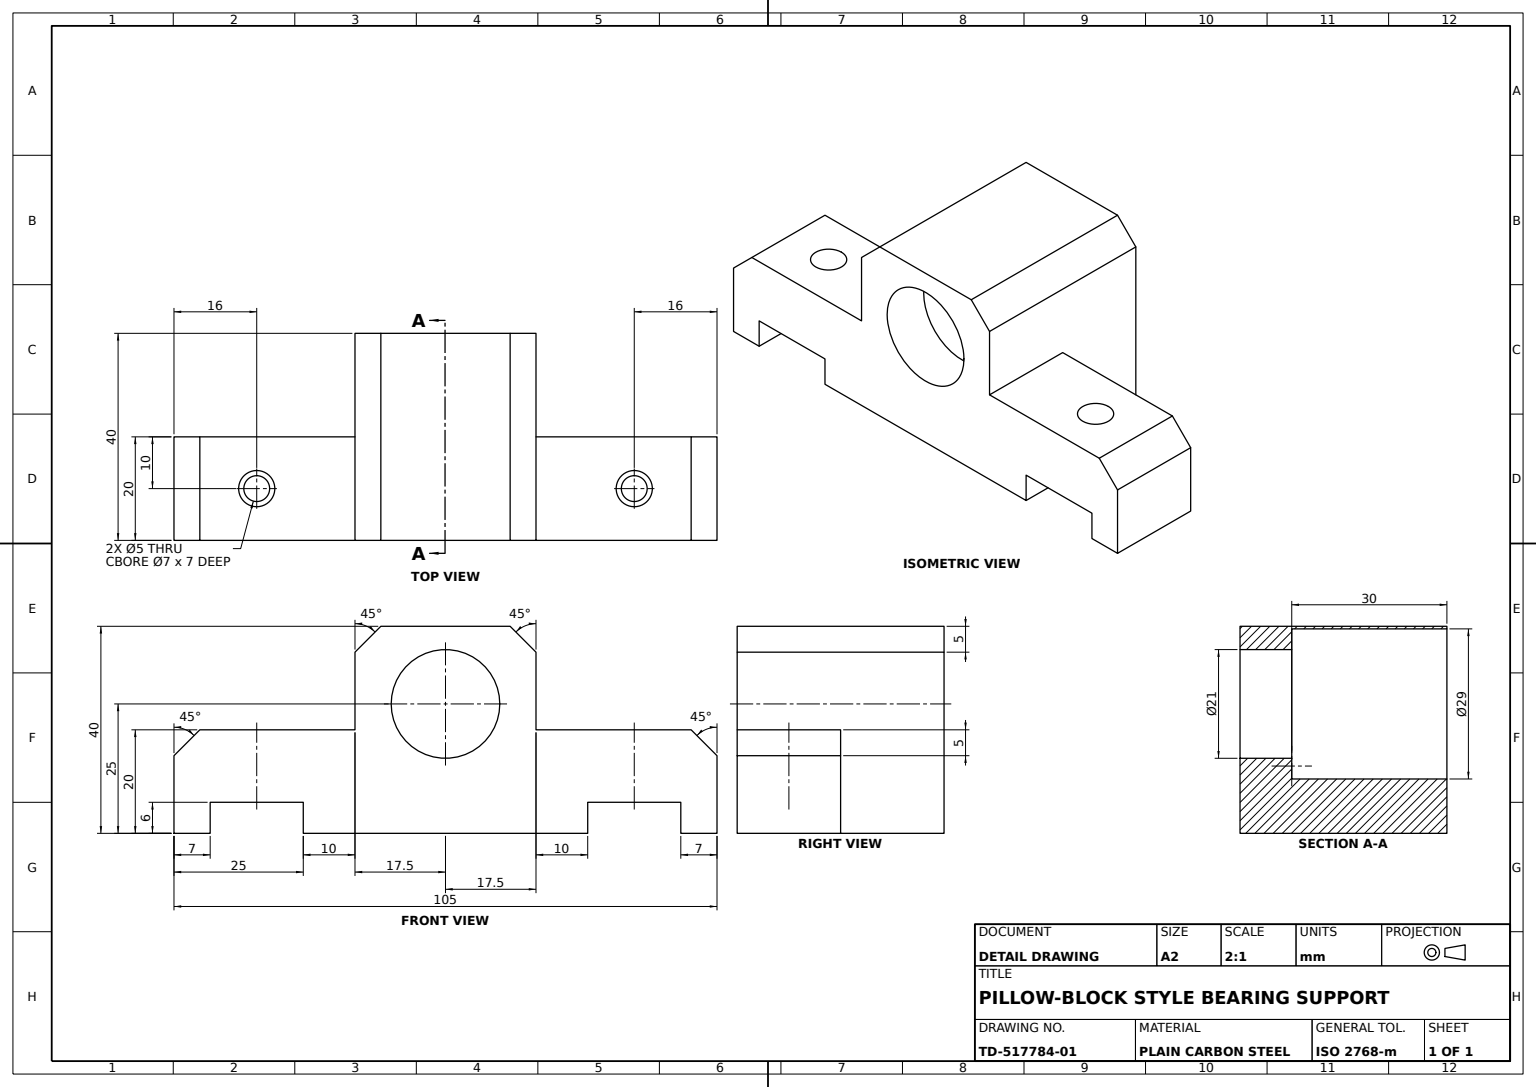
from build123d import *

# Parameters (mm, degrees)
BASE_BODY_DEPTH             = 40
MOUNTING_LUG_1_DEPTH        = 20
MOUNTING_LUG_2_DEPTH        = 20
LUG_2_BOTTOM_SLOT_PROFILE_W = 18
LUG_2_BOTTOM_SLOT_PROFILE_H = 6
LUG_2_BOTTOM_SLOT_DEPTH     = 20
LUG_1_BOTTOM_SLOT_PROFILE_W = 18
LUG_1_BOTTOM_SLOT_PROFILE_H = 6
LUG_1_BOTTOM_SLOT_DEPTH     = 20
LUG_2_HOLE_7_SKETCH_R       = 3.5
LUG_2_HOLE_7_DEPTH          = 7
LUG_2_HOLE_5_SKETCH_R       = 2.5
LUG_2_HOLE_5_DEPTH          = 7
LUG_1_HOLE_7_SKETCH_R       = 3.5
LUG_1_HOLE_7_DEPTH          = 7
LUG_1_HOLE_5_SKETCH_R       = 2.5
LUG_1_HOLE_5_DEPTH          = 7
BEARING_BORE_29_SKETCH_R    = 14.5
BEARING_BORE_29_DEPTH       = 30
THROUGH_BORE_21_SKETCH_R    = 10.5
THROUGH_BORE_21_DEPTH       = 87.02325267


with BuildPart() as part:
    # Base Body Profile → Base Body (new body)
    with BuildSketch(Plane.XY):
        Polygon((0, 0), (35, 0), (35, 35), (30, 40), (5, 40), (0, 35), align=None)
    extrude(amount=BASE_BODY_DEPTH)

    # Mounting Lug 1 Profile → Mounting Lug 1 (add)
    with BuildSketch(Plane.XY.offset(40)):
        Polygon((0, 0), (0, 20), (-19, 20), (-28, 20), (-30, 20), (-35, 15), (-35, 0), align=None)
    extrude(amount=-MOUNTING_LUG_1_DEPTH)

    # Mounting Lug 2 Profile → Mounting Lug 2 (add)
    with BuildSketch(Plane.XY.offset(40)):
        Polygon((35, 0), (35, 20), (54, 20), (63, 20), (65, 20), (70, 15), (70, 0), align=None)
    extrude(amount=-MOUNTING_LUG_2_DEPTH)

    # Lug 2 Bottom Slot Profile → Lug 2 Bottom Slot (cut)
    with BuildSketch(Plane(origin=(0, 0, 20), x_dir=(-1, 0, 0), z_dir=(0, 0, -1))):
        with Locations((-54, 3)):
            Rectangle(LUG_2_BOTTOM_SLOT_PROFILE_W, LUG_2_BOTTOM_SLOT_PROFILE_H)
    extrude(amount=-LUG_2_BOTTOM_SLOT_DEPTH, mode=Mode.SUBTRACT)

    # Lug 1 Bottom Slot Profile → Lug 1 Bottom Slot (cut)
    with BuildSketch(Plane(origin=(0, 0, 20), x_dir=(-1, 0, 0), z_dir=(0, 0, -1))):
        with Locations((19, 3)):
            Rectangle(LUG_1_BOTTOM_SLOT_PROFILE_W, LUG_1_BOTTOM_SLOT_PROFILE_H)
    extrude(amount=-LUG_1_BOTTOM_SLOT_DEPTH, mode=Mode.SUBTRACT)

    # Lug 2 Hole Ø7 Sketch → Lug 2 Hole Ø7 (cut)
    with BuildSketch(Plane(origin=(0, 20, 0), x_dir=(1, 0, 0), z_dir=(0, 1, 0))):
        with Locations(Location((54, -30, 0), (0, 0, 270))):
            Circle(LUG_2_HOLE_7_SKETCH_R)
    extrude(amount=-LUG_2_HOLE_7_DEPTH, mode=Mode.SUBTRACT)

    # Lug 2 Hole Ø5 Sketch → Lug 2 Hole Ø5 (cut)
    with BuildSketch(Plane(origin=(0, 13, 0), x_dir=(1, 0, 0), z_dir=(0, 1, 0))):
        with Locations(Location((54, -30, 0), (0, 0, 270))):
            Circle(LUG_2_HOLE_5_SKETCH_R)
    extrude(amount=-LUG_2_HOLE_5_DEPTH, mode=Mode.SUBTRACT)

    # Lug 1 Hole Ø7 Sketch → Lug 1 Hole Ø7 (cut)
    with BuildSketch(Plane(origin=(0, 20, 0), x_dir=(1, 0, 0), z_dir=(0, 1, 0))):
        with Locations(Location((-19, -30, 0), (0, 0, 270))):
            Circle(LUG_1_HOLE_7_SKETCH_R)
    extrude(amount=-LUG_1_HOLE_7_DEPTH, mode=Mode.SUBTRACT)

    # Lug 1 Hole Ø5 Sketch → Lug 1 Hole Ø5 (cut)
    with BuildSketch(Plane(origin=(0, 13, 0), x_dir=(1, 0, 0), z_dir=(0, 1, 0))):
        with Locations(Location((-19, -30, 0), (0, 0, 270))):
            Circle(LUG_1_HOLE_5_SKETCH_R)
    extrude(amount=-LUG_1_HOLE_5_DEPTH, mode=Mode.SUBTRACT)

    # Bearing Bore Ø29 Sketch → Bearing Bore Ø29 (cut)
    with BuildSketch(Plane(origin=(0, 0, 0), x_dir=(-1, 0, 0), z_dir=(0, 0, -1))):
        with Locations((-17.5, 25)):
            Circle(BEARING_BORE_29_SKETCH_R)
    extrude(amount=-BEARING_BORE_29_DEPTH, mode=Mode.SUBTRACT)

    # Through Bore Ø21 Sketch → Through Bore Ø21 (cut, through all)
    with BuildSketch(Plane(origin=(0, 0, 30), x_dir=(-1, 0, 0), z_dir=(0, 0, -1))):
        with Locations((-17.5, 25)):
            Circle(THROUGH_BORE_21_SKETCH_R)
    extrude(amount=-THROUGH_BORE_21_DEPTH, mode=Mode.SUBTRACT)


solid = part.part
